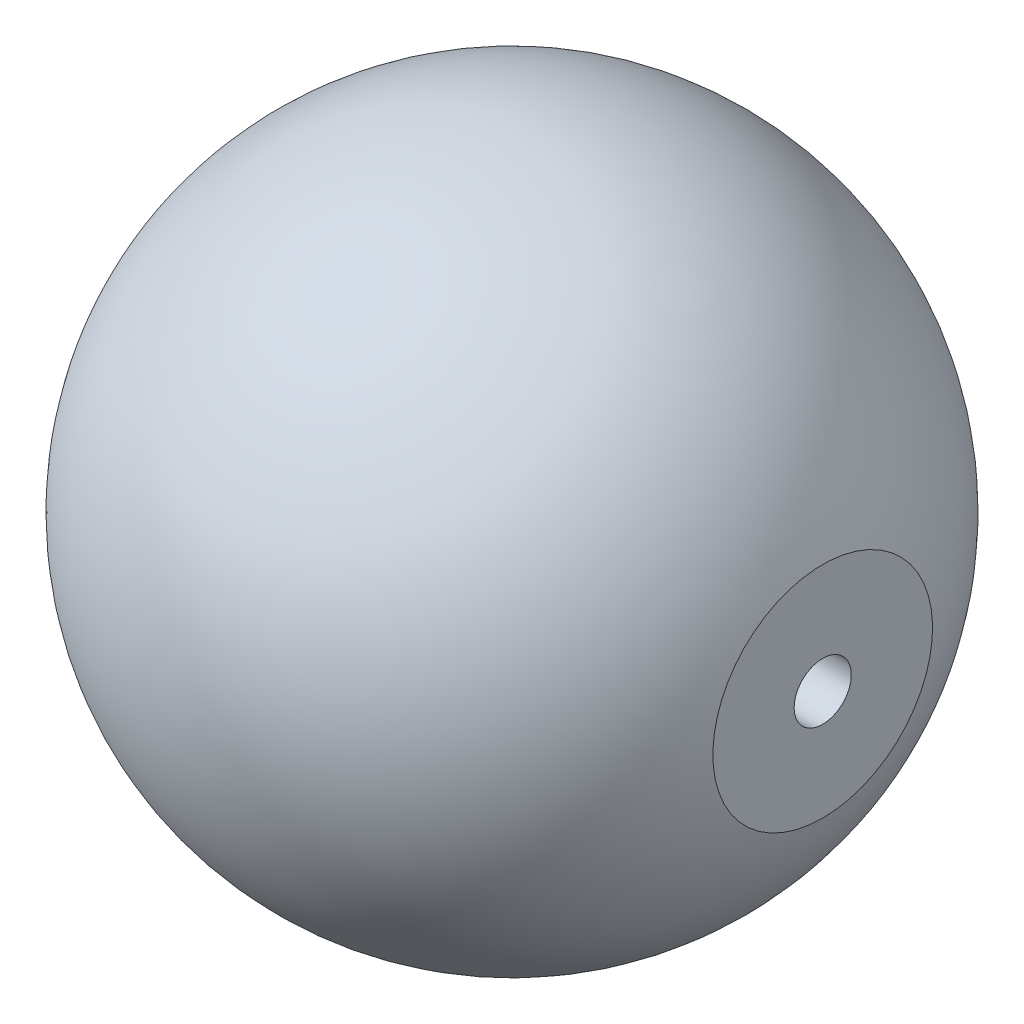
SolidWorks part; units mm, degrees
material "Plain Carbon Steel"
ref_plane "Front Plane" through (0, 0, 0) normal (0, 0, 1) x (1, 0, 0)
ref_plane "Top Plane" through (0, 0, 0) normal (0, 1, 0) x (1, 0, 0)
ref_plane "Right Plane" through (0, 0, 0) normal (1, 0, 0) x (0, 0, -1)
sketch "Knob Profile Sketch" plane through (0, 0, 0) normal (0, 0, 1) x (1, 0, 0)
  line L0 (-30, 0) -> (30, 0) construction
  line L1 (28.2843, -2.6) -> (29.8871, -2.6) construction
  line L2 (-28.2843, -2.6) -> (-28.2843, -10)
  line L3 (-28.2843, -2.6) -> (28.2843, -2.6)
  line L4 (0, 0) -> (0, 14.6496) construction
  line L5 (-28.2843, -2.6) -> (-28.2843, 0) construction
  line L6 (28.2843, -2.6) -> (28.2843, -10)
  line L7 (28.2843, -2.6) -> (28.2843, 0) construction
  line L8 (-28.2843, -2.6) -> (-29.8871, -2.6) construction
  arc A1 (-28.2843, -10) -> (28.2843, -10) centre (0, 0) ccw
  circle A2 centre (0, 0) radius 30 construction
  point P5 (-30, -2.6)
  point P6 (30, -2.6)
  dimension "D1" = 30
  dimension "D3" = 10
  dimension "D4" = 10
  dimension "D2" = 2.6
revolve "Ball Knob Revolve" add sketch "Knob Profile Sketch" angle 360 about L0
